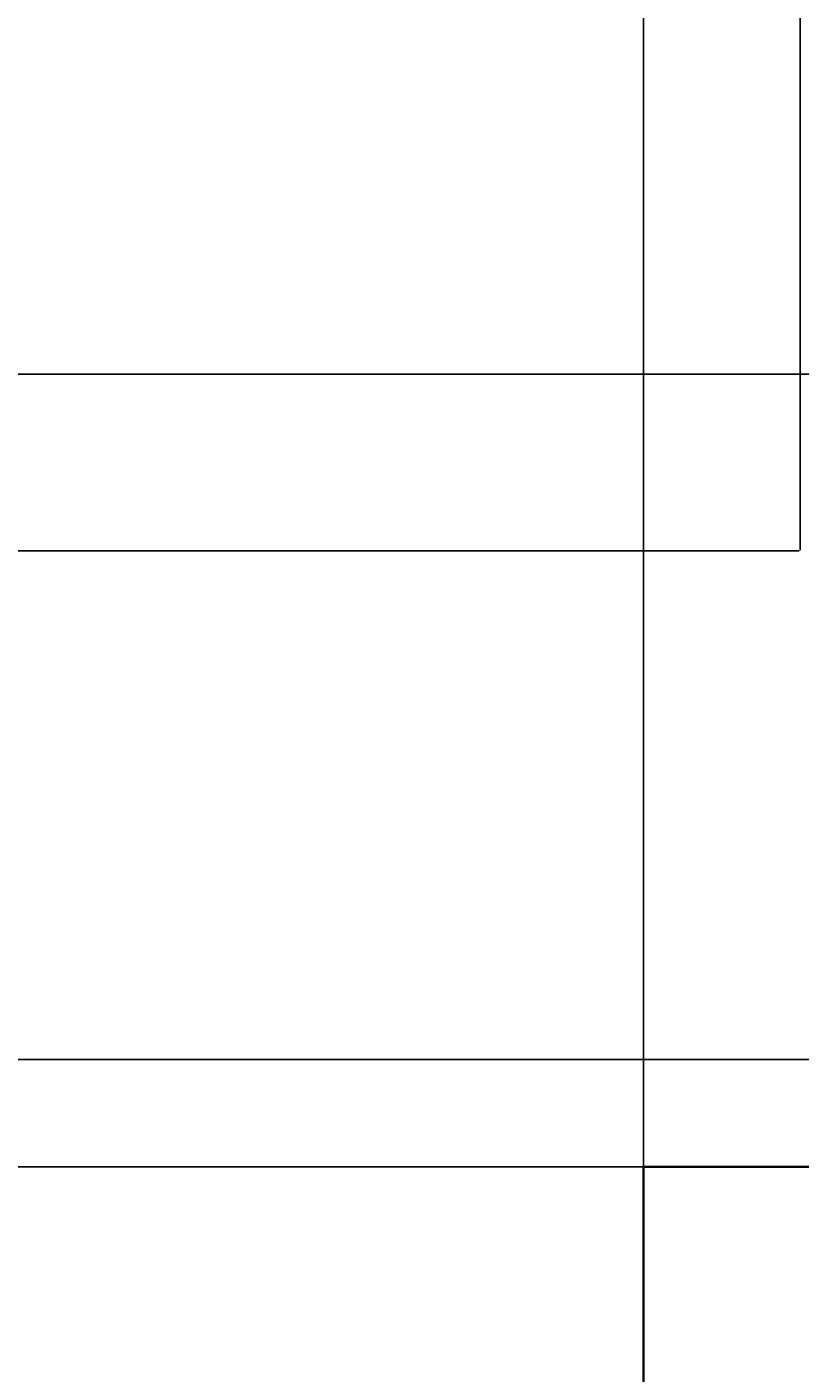
# Model space of a CAD drawing. Units: inches. Extents: x -13 to 809, y 112 to 656.
# Tile 27 of 55: x 47 to 107, y 446 to 551. Entities that reach past the tile are written whole.
import ezdxf

# ---------------------------------------------------------------- set-up
doc = ezdxf.new("R2010")
doc.units = ezdxf.units.IN
doc.header["$MEASUREMENT"] = 0
doc.layers.add('A-ANNO-DIMS', color=2, linetype='Continuous', lineweight=18)
doc.layers.add('A-ELEV', color=7, linetype='Continuous', lineweight=35)
doc.styles.get("Standard").update_dxf_attribs({"font": 'arial.ttf'})
doc.dimstyles.get("Standard").update_dxf_attribs({"dimtxt": 0.625, "dimasz": 0.18, "dimexe": 0.18, "dimexo": 0.0625, "dimgap": 0.09, "dimtad": 0, "dimtih": 1, "dimtoh": 1, "dimdec": 4, "dimzin": 0, "dimdsep": 46, "dimlunit": 4, "dimtxsty": 'Standard', "dimcen": 0.09, "dimadec": 0, "dimazin": 0, "dimtfac": 1, "dimtdec": 4, "dimtofl": 0, "dimtmove": 0, "dimatfit": 3, "dimfxl": 1, "dimtolj": 1, "dimtzin": 0, "dimarcsym": 0})

# ---------------------------------------------------------------- blocks, each defined once
blk = doc.blocks.new('*D22')
at = {"layer": 'A-ANNO-DIMS', "color": 0, "lineweight": -2, "transparency": 16777216}
for p, q in [((26.08, 210.58), (26.08, 655.96)), ((26.26, 655.78), (65.52, 655.78)), ((107.08, 655.78), (67.82, 655.78)), ((107.26, 510.58), (107.26, 655.96))]:
    blk.add_line(p, q, dxfattribs=at)
at = {"layer": 'A-ANNO-DIMS', "color": 0, "transparency": 16777216}
for points in [[(26.26, 655.81), (26.26, 655.75), (26.08, 655.78)], [(107.08, 655.81), (107.08, 655.75), (107.26, 655.78)]]:
    blk.add_solid(points, dxfattribs=at)
at = {"layer": 'Defpoints', "color": 0, "transparency": 16777216}
for p in [(107.26, 655.78), (107.26, 510.52), (26.08, 210.52)]:
    blk.add_point(p, dxfattribs=at)
at = {"layer": 'A-ANNO-DIMS', "color": 0, "transparency": 16777216, "insert": (66.67, 655.78), "char_height": 0.625, "attachment_point": 5}
blk.add_mtext('\\A1;81.18', dxfattribs=at)
blk = doc.blocks.new('*D23')
at = {"layer": 'A-ANNO-DIMS', "color": 0, "lineweight": -2, "transparency": 16777216}
for p, q in [((107.26, 510.58), (107.26, 655.96)), ((107.44, 655.78), (198.73, 655.78)), ((292.74, 655.78), (201.45, 655.78)), ((292.92, 569.3), (292.92, 655.96))]:
    blk.add_line(p, q, dxfattribs=at)
at = {"layer": 'A-ANNO-DIMS', "color": 0, "transparency": 16777216}
for points in [[(107.44, 655.81), (107.44, 655.75), (107.26, 655.78)], [(292.74, 655.81), (292.74, 655.75), (292.92, 655.78)]]:
    blk.add_solid(points, dxfattribs=at)
at = {"layer": 'Defpoints', "color": 0, "transparency": 16777216}
for p in [(292.92, 655.78), (292.92, 569.24), (107.26, 510.52)]:
    blk.add_point(p, dxfattribs=at)
at = {"layer": 'A-ANNO-DIMS', "color": 0, "transparency": 16777216, "insert": (200.09, 655.78), "char_height": 0.625, "attachment_point": 5}
blk.add_mtext('\\A1;185.66', dxfattribs=at)
blk = doc.blocks.new('*D34')
at = {"layer": 'A-ANNO-DIMS', "color": 0, "lineweight": -2, "transparency": 16777216}
for p, q in [((94.98, 462.52), (-12.1, 462.52)), ((-11.92, 462.34), (-11.92, 384.93)), ((-11.92, 306.7), (-11.92, 384.11)), ((94.98, 306.52), (-12.1, 306.52))]:
    blk.add_line(p, q, dxfattribs=at)
at = {"layer": 'A-ANNO-DIMS', "color": 0, "transparency": 16777216}
for points in [[(-11.95, 462.34), (-11.89, 462.34), (-11.92, 462.52)], [(-11.95, 306.7), (-11.89, 306.7), (-11.92, 306.52)]]:
    blk.add_solid(points, dxfattribs=at)
at = {"layer": 'Defpoints', "color": 0, "transparency": 16777216}
for p in [(-11.92, 462.52), (95.05, 462.52), (95.05, 306.52)]:
    blk.add_point(p, dxfattribs=at)
at = {"layer": 'A-ANNO-DIMS', "color": 0, "transparency": 16777216, "insert": (-11.92, 384.52), "char_height": 0.625, "attachment_point": 5}
blk.add_mtext('\\A1;156', dxfattribs=at)
blk = doc.blocks.new('*D35')
at = {"layer": 'A-ANNO-DIMS', "color": 0, "lineweight": -2, "transparency": 16777216}
for p, q in [((107.2, 510.52), (-12.1, 510.52)), ((-11.92, 510.34), (-11.92, 486.93)), ((-11.92, 462.7), (-11.92, 486.11)), ((107.2, 462.52), (-12.1, 462.52))]:
    blk.add_line(p, q, dxfattribs=at)
at = {"layer": 'A-ANNO-DIMS', "color": 0, "transparency": 16777216}
for points in [[(-11.95, 510.34), (-11.89, 510.34), (-11.92, 510.52)], [(-11.95, 462.7), (-11.89, 462.7), (-11.92, 462.52)]]:
    blk.add_solid(points, dxfattribs=at)
at = {"layer": 'Defpoints', "color": 0, "transparency": 16777216}
for p in [(-11.92, 510.52), (107.26, 510.52), (107.26, 462.52)]:
    blk.add_point(p, dxfattribs=at)
at = {"layer": 'A-ANNO-DIMS', "color": 0, "transparency": 16777216, "insert": (-11.92, 486.52), "char_height": 0.625, "attachment_point": 5}
blk.add_mtext('\\A1;48', dxfattribs=at)
blk = doc.blocks.new('*D36')
at = {"layer": 'A-ANNO-DIMS', "color": 0, "lineweight": -2, "transparency": 16777216}
for p, q in [((311.64, 569.24), (-12.1, 569.24)), ((-11.92, 569.06), (-11.92, 540.29)), ((-11.92, 510.7), (-11.92, 539.47)), ((107.2, 510.52), (-12.1, 510.52))]:
    blk.add_line(p, q, dxfattribs=at)
at = {"layer": 'A-ANNO-DIMS', "color": 0, "transparency": 16777216}
for points in [[(-11.95, 569.06), (-11.89, 569.06), (-11.92, 569.24)], [(-11.95, 510.7), (-11.89, 510.7), (-11.92, 510.52)]]:
    blk.add_solid(points, dxfattribs=at)
at = {"layer": 'Defpoints', "color": 0, "transparency": 16777216}
for p in [(-11.92, 569.24), (311.7, 569.24), (107.26, 510.52)]:
    blk.add_point(p, dxfattribs=at)
at = {"layer": 'A-ANNO-DIMS', "color": 0, "transparency": 16777216, "insert": (-11.92, 539.88), "char_height": 0.625, "attachment_point": 5}
blk.add_mtext('\\A1;58.72', dxfattribs=at)
blk = doc.blocks.new('*D39')
at = {"layer": 'A-ANNO-DIMS', "color": 0, "lineweight": -2, "transparency": 16777216}
for p, q in [((341.34, 524.28), (-12.1, 524.28)), ((-11.92, 524.1), (-11.92, 406.78)), ((-11.92, 288.63), (-11.92, 405.96)), ((341.34, 288.45), (-12.1, 288.45))]:
    blk.add_line(p, q, dxfattribs=at)
at = {"layer": 'A-ANNO-DIMS', "color": 0, "transparency": 16777216}
for points in [[(-11.95, 524.1), (-11.89, 524.1), (-11.92, 524.28)], [(-11.95, 288.63), (-11.89, 288.63), (-11.92, 288.45)]]:
    blk.add_solid(points, dxfattribs=at)
at = {"layer": 'Defpoints', "color": 0, "transparency": 16777216}
for p in [(-11.92, 524.28), (341.41, 524.28), (341.41, 288.45)]:
    blk.add_point(p, dxfattribs=at)
at = {"layer": 'A-ANNO-DIMS', "color": 0, "transparency": 16777216, "insert": (-11.92, 406.37), "char_height": 0.625, "attachment_point": 5}
blk.add_mtext('\\A1;235.83', dxfattribs=at)
blk = doc.blocks.new('*D43')
at = {"layer": 'A-ANNO-DIMS', "color": 0, "lineweight": -2, "transparency": 16777216}
for p, q in [((471.04, 470.88), (-12.1, 470.88)), ((-11.92, 470.7), (-11.92, 443.28)), ((-11.92, 415.04), (-11.92, 442.46)), ((471.04, 414.86), (-12.1, 414.86))]:
    blk.add_line(p, q, dxfattribs=at)
at = {"layer": 'A-ANNO-DIMS', "color": 0, "transparency": 16777216}
for points in [[(-11.95, 470.7), (-11.89, 470.7), (-11.92, 470.88)], [(-11.95, 415.04), (-11.89, 415.04), (-11.92, 414.86)]]:
    blk.add_solid(points, dxfattribs=at)
at = {"layer": 'Defpoints', "color": 0, "transparency": 16777216}
for p in [(-11.92, 470.88), (471.1, 470.88), (471.1, 414.86)]:
    blk.add_point(p, dxfattribs=at)
at = {"layer": 'A-ANNO-DIMS', "color": 0, "transparency": 16777216, "insert": (-11.92, 442.87), "char_height": 0.625, "attachment_point": 5}
blk.add_mtext('\\A1;56.02', dxfattribs=at)
blk = doc.blocks.new('*D95')
at = {"layer": 'A-ANNO-DIMS', "color": 0, "lineweight": -2, "transparency": 16777216}
for p, q in [((95.05, 462.58), (95.05, 655.96)), ((95.23, 655.78), (106.98, 655.78)), ((121.02, 655.78), (109.28, 655.78)), ((121.2, 452.63), (121.2, 655.96))]:
    blk.add_line(p, q, dxfattribs=at)
at = {"layer": 'A-ANNO-DIMS', "color": 0, "transparency": 16777216}
for points in [[(95.23, 655.81), (95.23, 655.75), (95.05, 655.78)], [(121.02, 655.81), (121.02, 655.75), (121.2, 655.78)]]:
    blk.add_solid(points, dxfattribs=at)
at = {"layer": 'Defpoints', "color": 0, "transparency": 16777216}
for p in [(121.2, 655.78), (95.05, 462.52), (121.2, 452.56)]:
    blk.add_point(p, dxfattribs=at)
at = {"layer": 'A-ANNO-DIMS', "color": 0, "transparency": 16777216, "insert": (108.13, 655.78), "char_height": 0.625, "attachment_point": 5}
blk.add_mtext('\\A1;26.16', dxfattribs=at)

msp = doc.modelspace()

# ---------------------------------------------------------------- linework, layer by layer
at = {"layer": 'A-ELEV'}
for p, q in [((95.0469, 318.5199), (95.0469, 462.5199)), ((95.0469, 462.5199), (337.5074, 462.5199))]:
    msp.add_line(p, q, dxfattribs=at)

# ---------------------------------------------------------------- dimensions: what is measured, and where the dimension line sits
at = {"layer": 'A-ANNO-DIMS'}
for base, p1, p2, picture, middle in [((107.2588, 655.7828), (26.0809, 210.5199), (107.2588, 510.5199), '*D22', (66.6698, 655.7828)), ((121.2048, 655.7828), (95.0469, 462.5199), (121.2048, 452.5629), '*D95', (108.1258, 655.7828)), ((292.923, 655.7828), (107.2588, 510.5199), (292.923, 569.2414), '*D23', (200.0909, 655.7828))]:
    dim = msp.add_linear_dim(base=base, p1=p1, p2=p2, dimstyle='Standard', override={"dimdec": 2, "dimlfac": 1, "dimrnd": 0, "dimzin": 0, "dimdsep": 46, "dimlunit": 2}, dxfattribs=at)
    dim.commit()
    dim.dimension.update_dxf_attribs({"geometry": picture, "text_midpoint": middle})
for base, p1, p2, override, picture, middle in [((-11.9191, 569.2414), (107.2588, 510.5199), (311.6991, 569.2414), {"dimdec": 2, "dimlfac": 1, "dimrnd": 0, "dimzin": 0, "dimdsep": 46, "dimlunit": 2}, '*D36', (-11.9191, 539.8806)), ((-11.9191, 524.281), (341.4072, 288.4508), (341.4072, 524.281), {"dimdec": 2, "dimlfac": 1, "dimrnd": 0, "dimzin": 0, "dimdsep": 46, "dimlunit": 2}, '*D39', (-11.9191, 406.3659)), ((-11.9191, 510.5199), (107.2588, 462.5199), (107.2588, 510.5199), {"dimdec": 0, "dimlfac": 1, "dimrnd": 0, "dimzin": 0, "dimdsep": 46, "dimlunit": 2}, '*D35', (-11.9191, 486.5199)), ((-11.9191, 470.8765), (471.0998, 414.8594), (471.0998, 470.8765), {"dimdec": 2, "dimlfac": 1, "dimrnd": 0, "dimzin": 0, "dimdsep": 46, "dimlunit": 2}, '*D43', (-11.9191, 442.8679)), ((-11.9191, 462.5199), (95.0469, 306.5199), (95.0469, 462.5199), {"dimdec": 0, "dimlfac": 1, "dimrnd": 0, "dimzin": 0, "dimdsep": 46, "dimlunit": 2}, '*D34', (-11.9191, 384.5199))]:
    dim = msp.add_linear_dim(base=base, p1=p1, p2=p2, angle=90, dimstyle='Standard', override=override, dxfattribs=at)
    dim.commit()
    dim.dimension.update_dxf_attribs({"geometry": picture, "text_midpoint": middle})

doc.saveas('drawing.dxf')
